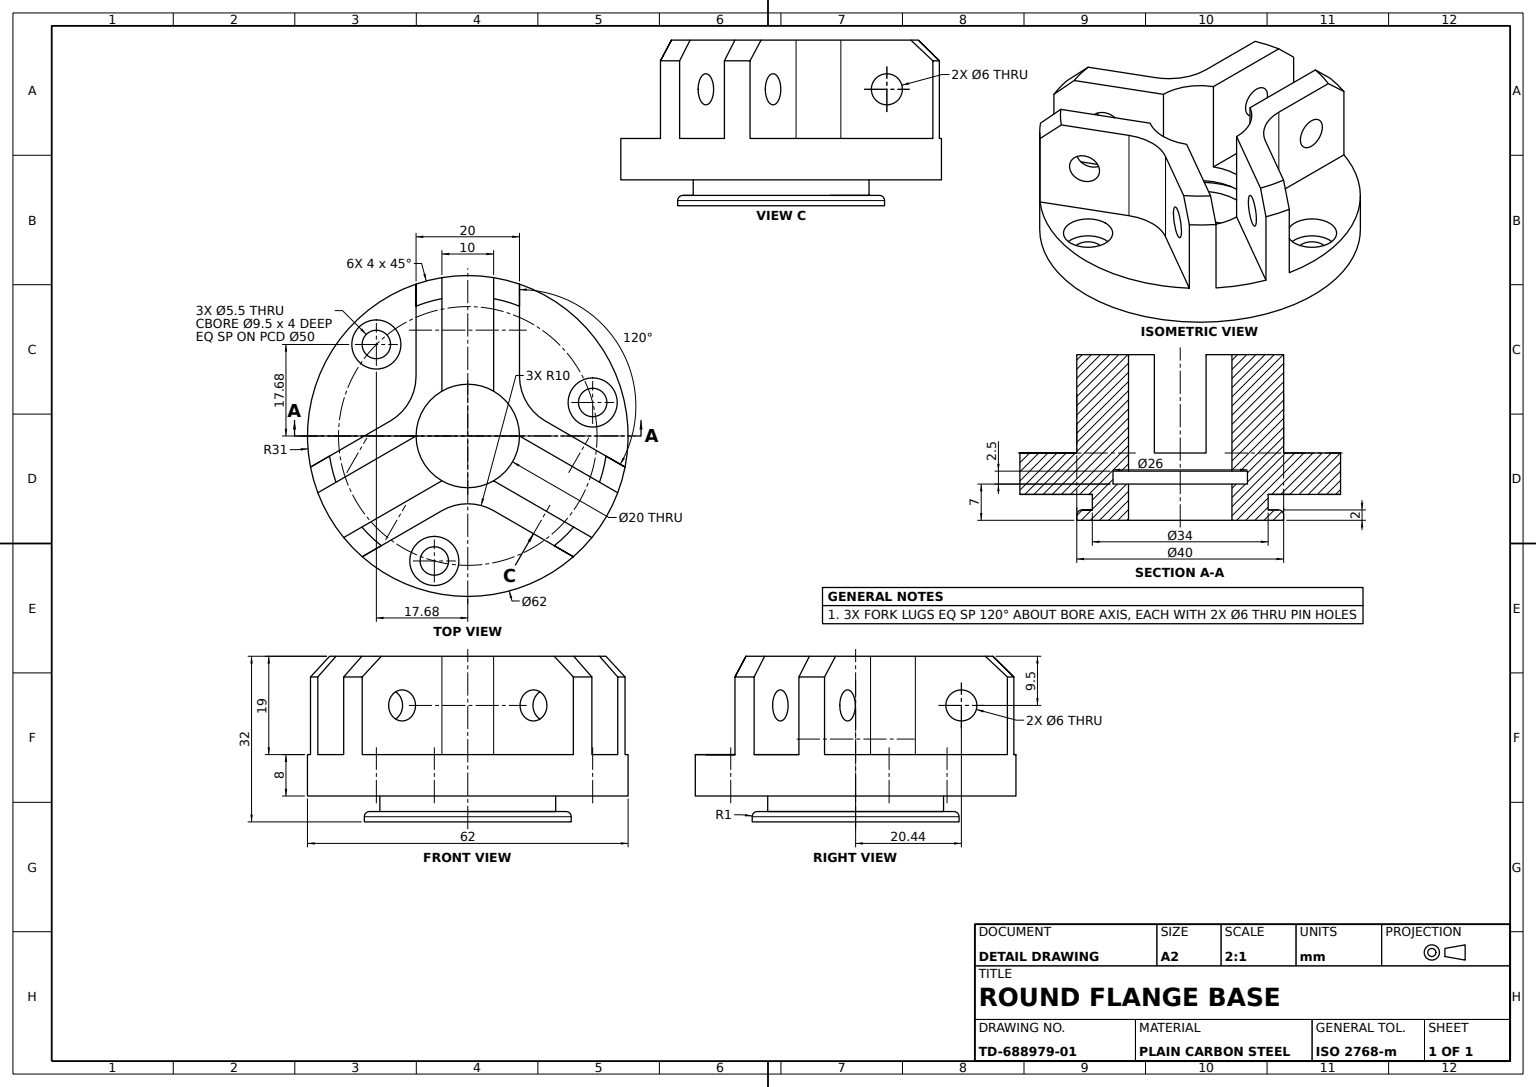
from build123d import *
from build123d.topology import SkipClean

# Parameters (mm, degrees)
BASE_FLANGE_SKETCH_R                        = 31
BASE_FLANGE_62_DEPTH                        = 8
HUB_BOSS_SKETCH_R                           = 17
HUB_BOSS_34_DEPTH                           = 3
HUB_COLLAR_SKETCH_R                         = 20
HUB_COLLAR_40_DEPTH                         = 2
HUB_COLLAR_FILLET_R1_R                      = 1
CENTRAL_BORE_PROFILE_W                      = 13
CENTRAL_BORE_PROFILE_H                      = 2.5
MOUNTING_HOLES_3X_5_5_CBORE_9_5_D           = 5.5
MOUNTING_HOLES_3X_5_5_CBORE_9_5_DEPTH       = 8.774964387
MOUNTING_HOLES_3X_5_5_CBORE_9_5_CBORE_D     = 9.5
MOUNTING_HOLES_3X_5_5_CBORE_9_5_CBORE_DEPTH = 4
FORK_LUGS_DEPTH                             = 19
SKETCH8_6_R                                 = 10
FORK_LUG_RELIEF_CUT_DEPTH                   = 48.780749262
LUG_1_PIN_HOLE_SKETCH_R                     = 3
LUG_1_PIN_HOLE_6_DEPTH                      = 60.982795453
LUG_2_PIN_HOLE_SKETCH_R                     = 3
LUG_2_PIN_HOLE_6_DEPTH                      = 60.982795453
LUG_3_PIN_HOLE_SKETCH_R                     = 3
LUG_3_PIN_HOLE_6_DEPTH                      = 59.060313468
FORK_LUG_CHAMFER_4X45_SIZE                  = 4


with BuildPart() as part:
    # Base Flange Sketch → Base Flange _62 (new body)
    with BuildSketch(Plane(origin=(0, 0, 0), x_dir=(1, 0, 0), z_dir=(0, 1, 0))):
        with Locations(Location((0, 0, 0), (0, 0, 270))):
            Circle(BASE_FLANGE_SKETCH_R)
    extrude(amount=BASE_FLANGE_62_DEPTH)

    # Hub Boss Sketch → Hub Boss _34 (add)
    with BuildSketch(Plane.XZ):
        with Locations(Location((0, 0, 0), (0, 0, 270))):
            Circle(HUB_BOSS_SKETCH_R)
    extrude(amount=HUB_BOSS_34_DEPTH)

    # Hub Collar Sketch → Hub Collar _40 (add)
    with BuildSketch(Plane.XZ.offset(3)):
        with Locations(Location((0, 0, 0), (0, 0, 270))):
            Circle(HUB_COLLAR_SKETCH_R)
    extrude(amount=HUB_COLLAR_40_DEPTH)

    # Hub Collar Fillet R1
    hub_collar_fillet_r1_edges = [part.edges().sort_by_distance(p)[0] for p in [
        (0, -3, 20),
    ]]
    fillet(hub_collar_fillet_r1_edges, radius=HUB_COLLAR_FILLET_R1_R)

    # Central Bore Profile → Central Bore (revolve, cut)
    with BuildSketch(Plane(origin=(0, 0, 0), x_dir=(0, 0, -1), z_dir=(1, 0, 0)), mode=Mode.PRIVATE) as central_bore_sk:
        with Locations((-6.5, 3.25)):
            Rectangle(CENTRAL_BORE_PROFILE_W, CENTRAL_BORE_PROFILE_H)
    revolve(central_bore_sk.sketch.rotate(Axis((0, 2, 0), (0, 1, 0)), 180), axis=Axis((0, 2, 0), (0, 1, 0)), mode=Mode.SUBTRACT)

    # Mounting Holes 3x_5.5 CBore _9.5
    with Locations(Plane(origin=(0, 8, 0), x_dir=(1, 0, 0), z_dir=(0, 1, 0))):
        with Locations((-17.67766953, 17.67766953), (24.148145657, 6.470476128), (-6.470476128, -24.148145657)):
            CounterBoreHole(MOUNTING_HOLES_3X_5_5_CBORE_9_5_D / 2, MOUNTING_HOLES_3X_5_5_CBORE_9_5_CBORE_D / 2, MOUNTING_HOLES_3X_5_5_CBORE_9_5_CBORE_DEPTH, depth=MOUNTING_HOLES_3X_5_5_CBORE_9_5_DEPTH)

    # Fork Lugs Sketch → Fork Lugs (add)
    with BuildSketch(Plane(origin=(0, 8, 0), x_dir=(1, 0, 0), z_dir=(0, 1, 0))):
        with BuildLine():
            Line((5, 30.594117082), (5, 8.660254038))
            ThreePointArc((5, 8.660254038), (8.660254038, 5), (10, 0))
            Line((10, 0), (28.995282599, -10.966931522))
            ThreePointArc((28.995282599, -10.966931522), (29.806622049, -8.518525814), (30.411611519, -6.011146713))
            Line((30.411611519, -6.011146713), (15, 2.886751346))
            ThreePointArc((15, 2.886751346), (11.339745962, 6.547005384), (10, 11.547005384))
            Line((10, 11.547005384), (10, 29.342801502))
            ThreePointArc((10, 29.342801502), (7.526051267, 30.072554802), (5, 30.594117082))
        make_face()
        with BuildLine():
            ThreePointArc((-10, 0), (-8.660254038, 5), (-5, 8.660254038))
            Line((-5, 8.660254038), (-5, 30.594117082))
            ThreePointArc((-5, 30.594117082), (-7.526051267, 30.072554802), (-10, 29.342801502))
            Line((-10, 29.342801502), (-10, 11.547005384))
            ThreePointArc((-10, 11.547005384), (-11.339745962, 6.547005384), (-15, 2.886751346))
            Line((-15, 2.886751346), (-30.411611519, -6.011146713))
            ThreePointArc((-30.411611519, -6.011146713), (-29.806622049, -8.518525814), (-28.995282599, -10.966931522))
            Line((-28.995282599, -10.966931522), (-10, 0))
        make_face()
        with BuildLine():
            Line((23.995282599, -19.62718556), (5, -8.660254038))
            ThreePointArc((5, -8.660254038), (0, -10), (-5, -8.660254038))
            Line((-5, -8.660254038), (-23.995282599, -19.62718556))
            ThreePointArc((-23.995282599, -19.62718556), (-22.280570782, -21.554028988), (-20.411611519, -23.331654789))
            Line((-20.411611519, -23.331654789), (-5, -14.43375673))
            ThreePointArc((-5, -14.43375673), (0, -13.094010768), (5, -14.43375673))
            Line((5, -14.43375673), (20.411611519, -23.331654789))
            ThreePointArc((20.411611519, -23.331654789), (22.280570782, -21.554028988), (23.995282599, -19.62718556))
        make_face()
    extrude(amount=FORK_LUGS_DEPTH)

    # Sketch8_6 → Fork Lug Relief Cut (cut, through all)
    with SkipClean():  # the faces are left unmerged after this step: merging them gives an invalid solid
        with BuildSketch(Plane(origin=(0, 8, 0), x_dir=(1, 0, 0), z_dir=(0, 1, 0))):
            with Locations(Location((0, 0, 0), (0, 0, 90))):
                Circle(SKETCH8_6_R)
        extrude(amount=-FORK_LUG_RELIEF_CUT_DEPTH, mode=Mode.SUBTRACT)

    # Lug 1 Pin Hole Sketch → Lug 1 Pin Hole _6 (cut, through all)
    with SkipClean():  # the faces are left unmerged after this step: merging them gives an invalid solid
        with BuildSketch(Plane(origin=(-5, 0, 8.660254038), x_dir=(0.8660254037844363, 0, 0.5000000000000043), z_dir=(-0.5000000000000042, 0, 0.8660254037844362))):
            with Locations((20.444903443, 17.5)):
                Circle(LUG_1_PIN_HOLE_SKETCH_R)
        extrude(amount=-LUG_1_PIN_HOLE_6_DEPTH, mode=Mode.SUBTRACT)

    # Lug 2 Pin Hole Sketch → Lug 2 Pin Hole _6 (cut, through all)
    with SkipClean():  # the faces are left unmerged after this step: merging them gives an invalid solid
        with BuildSketch(Plane(origin=(-5, 0, -8.660254038), x_dir=(-0.8660254037844363, 0, 0.5000000000000042), z_dir=(-0.5000000000000042, 0, -0.8660254037844363))):
            with Locations(Location((20.444903443, 17.5, 0), (0, 0, 180))):
                Circle(LUG_2_PIN_HOLE_SKETCH_R)
        extrude(amount=-LUG_2_PIN_HOLE_6_DEPTH, mode=Mode.SUBTRACT)

    # Lug 3 Pin Hole Sketch → Lug 3 Pin Hole _6 (cut, through all)
    with SkipClean():  # the faces are left unmerged after this step: merging them gives an invalid solid
        with BuildSketch(Plane(origin=(10, 0, 0), x_dir=(0, 0, -1), z_dir=(1, 0, 0))):
            with Locations(Location((20.444903443, 17.5, 0), (0, 0, 180))):
                Circle(LUG_3_PIN_HOLE_SKETCH_R)
        extrude(amount=-LUG_3_PIN_HOLE_6_DEPTH, mode=Mode.SUBTRACT)

    # Fork Lug Chamfer 4x45
    fork_lug_chamfer_4x45_edges = [part.edges().sort_by_distance(p)[0] for p in [
        (7.526051267, 27, -30.072554802),
        (29.806622049, 27, 8.518525814),
        (-29.806622049, 27, 8.518525814),
        (-7.526051267, 27, -30.072554802),
        (22.280570782, 27, 21.554028988),
        (-22.280570782, 27, 21.554028988),
    ]]
    chamfer(fork_lug_chamfer_4x45_edges, length=FORK_LUG_CHAMFER_4X45_SIZE)


solid = part.part
